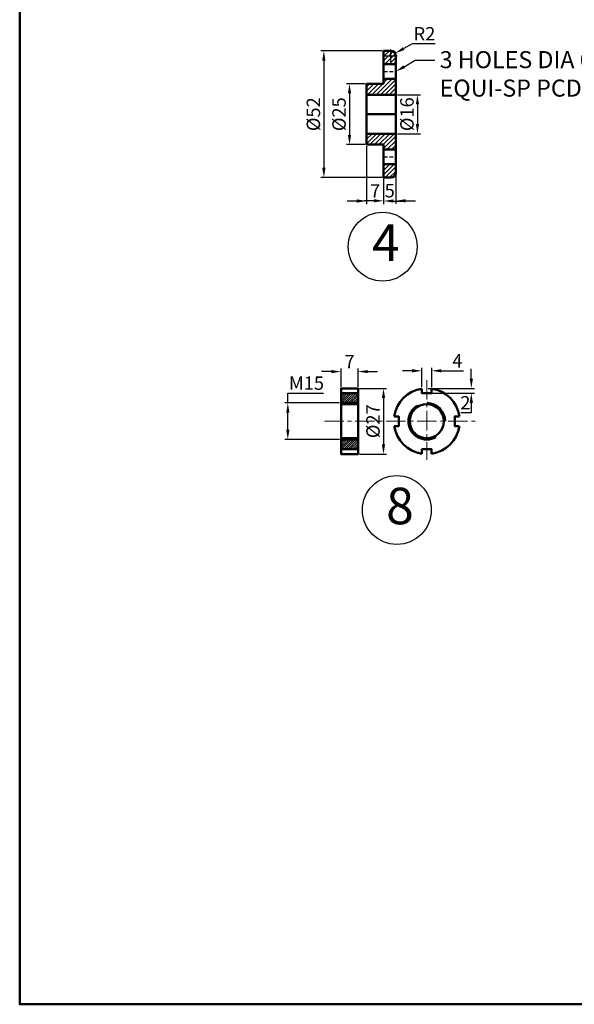
# Model space of a CAD drawing. Units: millimetres. Extents: x -3 to 930, y -425 to 322.
# Tile 1 of 5: x -3 to 225, y -425 to -21. Entities that reach past the tile are written whole.
import ezdxf
from ezdxf import colors
from ezdxf.entities.mleader import LeaderData, LeaderLine
from ezdxf.math import Vec2, Vec3

# ---------------------------------------------------------------- set-up
doc = ezdxf.new("R2010")
doc.units = ezdxf.units.MM
doc.header["$LTSCALE"] = 0.5
doc.linetypes.add('CENTER', pattern=[50.8, 31.75, -6.35, 6.35, -6.35])
doc.linetypes.add('HIDDEN', pattern=[9.525, 6.35, -3.175])
for name, color, linetype, lineweight in [('M-ANNO-SYMB', 3, 'Continuous', 25), ('M-CNTR', 1, 'CENTER', 18), ('M-DIMS', 2, 'Continuous', 25), ('M-HATC', 8, 'Continuous', 18), ('M-HIDN', 4, 'HIDDEN', 25), ('M-OUTL', 7, 'Continuous', 50), ('M-TEXT', 3, 'Continuous', 25)]:
    doc.layers.add(name, color=color, linetype=linetype, lineweight=lineweight)
doc.styles.get("Standard").update_dxf_attribs({"font": 'arial.ttf'})
doc.dimstyles.new('ISO-25', dxfattribs={"dimtxt": 5.5, "dimasz": 4, "dimexe": 1.25, "dimexo": 0.625, "dimtad": 1, "dimtoh": 1, "dimdec": 0, "dimtxsty": 'Standard', "dimcen": 2.5, "dimadec": 0, "dimazin": 0, "dimtfac": 1, "dimtdec": 0, "dimtofl": 0, "dimtmove": 0, "dimatfit": 3, "dimfxl": 1, "dimarcsym": 0})
pattern_1 = [(45, (-143.9728, 27.2126), (-0.8980256, 0.8980256), [])]

# ---------------------------------------------------------------- blocks, each defined once
blk = doc.blocks.new('*D43')
at = {"layer": 'Defpoints', "color": 0, "ltscale": 0.5, "transparency": 16777216}
for p in [(146.67, -33.61), (122.15, -85.61), (146.67, -85.61)]:
    blk.add_point(p, dxfattribs=at)
at = {"layer": 'M-DIMS', "color": 0, "lineweight": -2, "ltscale": 0.5, "transparency": 16777216}
for p, q in [((146.04, -33.61), (120.9, -33.61)), ((122.15, -37.61), (122.15, -81.61)), ((146.04, -85.61), (120.9, -85.61))]:
    blk.add_line(p, q, dxfattribs=at)
at = {"layer": 'M-DIMS', "color": 0, "ltscale": 0.5, "transparency": 16777216}
for points in [[(121.48, -37.61), (122.82, -37.61), (122.15, -33.61)], [(121.48, -81.61), (122.82, -81.61), (122.15, -85.61)]]:
    blk.add_solid(points, dxfattribs=at)
at = {"layer": 'M-DIMS', "color": 0, "ltscale": 0.5, "transparency": 16777216, "insert": (118.56, -59.61), "char_height": 5.5, "attachment_point": 5, "rotation": 90}
blk.add_mtext('%%C52', dxfattribs=at)
blk = doc.blocks.new('*D44')
at = {"layer": 'Defpoints', "color": 0, "ltscale": 0.5, "transparency": 16777216}
for p in [(139.67, -47.11), (132.67, -72.11), (139.67, -72.11)]:
    blk.add_point(p, dxfattribs=at)
at = {"layer": 'M-DIMS', "color": 0, "lineweight": -2, "ltscale": 0.5, "transparency": 16777216}
for p, q in [((139.04, -47.11), (131.42, -47.11)), ((132.67, -51.11), (132.67, -68.11)), ((139.04, -72.11), (131.42, -72.11))]:
    blk.add_line(p, q, dxfattribs=at)
at = {"layer": 'M-DIMS', "color": 0, "ltscale": 0.5, "transparency": 16777216}
for points in [[(132, -51.11), (133.34, -51.11), (132.67, -47.11)], [(132, -68.11), (133.34, -68.11), (132.67, -72.11)]]:
    blk.add_solid(points, dxfattribs=at)
at = {"layer": 'M-DIMS', "color": 0, "ltscale": 0.5, "transparency": 16777216, "insert": (129.08, -59.61), "char_height": 5.5, "attachment_point": 5, "rotation": 90}
blk.add_mtext('%%C25', dxfattribs=at)
blk = doc.blocks.new('*D45')
at = {"layer": 'Defpoints', "color": 0, "ltscale": 0.5, "transparency": 16777216}
for p in [(151.67, -51.61), (151.67, -67.61), (160.53, -67.61)]:
    blk.add_point(p, dxfattribs=at)
at = {"layer": 'M-DIMS', "color": 0, "lineweight": -2, "ltscale": 0.5, "transparency": 16777216}
for p, q in [((152.29, -51.61), (161.78, -51.61)), ((160.53, -55.61), (160.53, -63.61)), ((152.29, -67.61), (161.78, -67.61))]:
    blk.add_line(p, q, dxfattribs=at)
at = {"layer": 'M-DIMS', "color": 0, "ltscale": 0.5, "transparency": 16777216}
for points in [[(159.87, -55.61), (161.2, -55.61), (160.53, -51.61)], [(159.87, -63.61), (161.2, -63.61), (160.53, -67.61)]]:
    blk.add_solid(points, dxfattribs=at)
at = {"layer": 'M-DIMS', "color": 0, "ltscale": 0.5, "transparency": 16777216, "insert": (156.95, -59.61), "char_height": 5.5, "attachment_point": 5, "rotation": 90}
blk.add_mtext('%%C16', dxfattribs=at)
blk = doc.blocks.new('*D46')
at = {"layer": 'Defpoints', "color": 0, "ltscale": 0.5, "transparency": 16777216}
for p in [(139.67, -72.11), (146.67, -72.11), (146.67, -95.23)]:
    blk.add_point(p, dxfattribs=at)
at = {"layer": 'M-DIMS', "color": 0, "lineweight": -2, "ltscale": 0.5, "transparency": 16777216}
for p, q in [((139.67, -72.73), (139.67, -96.48)), ((146.67, -72.73), (146.67, -96.48)), ((135.67, -95.23), (131.67, -95.23)), ((150.67, -95.23), (154.67, -95.23))]:
    blk.add_line(p, q, dxfattribs=at)
at = {"layer": 'M-DIMS', "color": 0, "ltscale": 0.5, "transparency": 16777216}
for points in [[(135.67, -94.56), (135.67, -95.9), (139.67, -95.23)], [(150.67, -94.56), (150.67, -95.9), (146.67, -95.23)]]:
    blk.add_solid(points, dxfattribs=at)
at = {"layer": 'M-DIMS', "color": 0, "ltscale": 0.5, "transparency": 16777216, "insert": (143.17, -91.86), "char_height": 5.5, "attachment_point": 5}
blk.add_mtext('7', dxfattribs=at)
blk = doc.blocks.new('*D47')
at = {"layer": 'Defpoints', "color": 0, "ltscale": 0.5, "transparency": 16777216}
for p in [(146.67, -74.11), (151.67, -74.11), (151.67, -95.15)]:
    blk.add_point(p, dxfattribs=at)
at = {"layer": 'M-DIMS', "color": 0, "lineweight": -2, "ltscale": 0.5, "transparency": 16777216}
for p, q in [((146.67, -74.73), (146.67, -96.4)), ((151.67, -74.73), (151.67, -96.4)), ((142.67, -95.15), (138.67, -95.15)), ((155.67, -95.15), (159.67, -95.15))]:
    blk.add_line(p, q, dxfattribs=at)
at = {"layer": 'M-DIMS', "color": 0, "ltscale": 0.5, "transparency": 16777216}
for points in [[(142.67, -94.48), (142.67, -95.81), (146.67, -95.15)], [(155.67, -94.48), (155.67, -95.81), (151.67, -95.15)]]:
    blk.add_solid(points, dxfattribs=at)
at = {"layer": 'M-DIMS', "color": 0, "ltscale": 0.5, "transparency": 16777216, "insert": (149.17, -91.72), "char_height": 5.5, "attachment_point": 5}
blk.add_mtext('5', dxfattribs=at)
blk = doc.blocks.new('*D48')
at = {"layer": 'Defpoints', "color": 0, "ltscale": 0.5, "transparency": 16777216}
for p in [(149.67, -35.61), (151.41, -34.62)]:
    blk.add_point(p, dxfattribs=at)
at = {"layer": 'M-DIMS', "color": 0, "lineweight": -2, "ltscale": 0.5, "transparency": 16777216}
for p, q in [((158.38, -30.7), (154.89, -32.66)), ((167.82, -30.7), (158.38, -30.7)), ((147.17, -35.61), (152.17, -35.61)), ((149.67, -38.11), (149.67, -33.11))]:
    blk.add_line(p, q, dxfattribs=at)
at = {"layer": 'M-DIMS', "color": 0, "ltscale": 0.5, "transparency": 16777216}
blk.add_solid([(154.57, -32.08), (155.22, -33.24), (151.41, -34.62)], dxfattribs=at)
at = {"layer": 'M-DIMS', "color": 0, "ltscale": 0.5, "transparency": 16777216, "insert": (163.41, -27.31), "char_height": 5.5, "attachment_point": 5}
blk.add_mtext('R2', dxfattribs=at)
blk = doc.blocks.new('*D61')
at = {"layer": 'Defpoints', "color": 0, "ltscale": 0.5, "transparency": 16777216}
for p in [(107.36, -178.11), (129.18, -178.11), (129.18, -193.11)]:
    blk.add_point(p, dxfattribs=at)
at = {"layer": 'M-DIMS', "color": 0, "lineweight": -2, "ltscale": 0.5, "transparency": 16777216}
for p, q in [((107.36, -178.11), (107.36, -174.11)), ((107.36, -174.11), (122.06, -174.11)), ((128.56, -178.11), (106.11, -178.11)), ((107.36, -189.11), (107.36, -182.11)), ((128.56, -193.11), (106.11, -193.11))]:
    blk.add_line(p, q, dxfattribs=at)
at = {"layer": 'M-DIMS', "color": 0, "ltscale": 0.5, "transparency": 16777216}
for points in [[(106.7, -182.11), (108.03, -182.11), (107.36, -178.11)], [(106.7, -189.11), (108.03, -189.11), (107.36, -193.11)]]:
    blk.add_solid(points, dxfattribs=at)
at = {"layer": 'M-DIMS', "color": 0, "ltscale": 0.5, "transparency": 16777216, "insert": (115.02, -170.68), "char_height": 5.5, "attachment_point": 5}
blk.add_mtext('M15', dxfattribs=at)
blk = doc.blocks.new('*D62')
at = {"layer": 'Defpoints', "color": 0, "ltscale": 0.5, "transparency": 16777216}
for p in [(136.18, -165.24), (129.18, -172.11), (136.18, -172.11)]:
    blk.add_point(p, dxfattribs=at)
at = {"layer": 'M-DIMS', "color": 0, "lineweight": -2, "ltscale": 0.5, "transparency": 16777216}
for p, q in [((125.18, -165.24), (121.18, -165.24)), ((129.18, -171.49), (129.18, -163.99)), ((136.18, -171.49), (136.18, -163.99)), ((140.18, -165.24), (144.18, -165.24))]:
    blk.add_line(p, q, dxfattribs=at)
at = {"layer": 'M-DIMS', "color": 0, "ltscale": 0.5, "transparency": 16777216}
for points in [[(125.18, -164.57), (125.18, -165.9), (129.18, -165.24)], [(140.18, -164.57), (140.18, -165.9), (136.18, -165.24)]]:
    blk.add_solid(points, dxfattribs=at)
at = {"layer": 'M-DIMS', "color": 0, "ltscale": 0.5, "transparency": 16777216, "insert": (132.68, -161.86), "char_height": 5.5, "attachment_point": 5}
blk.add_mtext('7', dxfattribs=at)
blk = doc.blocks.new('*D63')
at = {"layer": 'Defpoints', "color": 0, "ltscale": 0.5, "transparency": 16777216}
for p in [(136.18, -172.11), (136.18, -199.11), (146.6, -199.11)]:
    blk.add_point(p, dxfattribs=at)
at = {"layer": 'M-DIMS', "color": 0, "lineweight": -2, "ltscale": 0.5, "transparency": 16777216}
for p, q in [((136.81, -172.11), (147.85, -172.11)), ((146.6, -176.11), (146.6, -195.11)), ((136.81, -199.11), (147.85, -199.11))]:
    blk.add_line(p, q, dxfattribs=at)
at = {"layer": 'M-DIMS', "color": 0, "ltscale": 0.5, "transparency": 16777216}
for points in [[(145.94, -176.11), (147.27, -176.11), (146.6, -172.11)], [(145.94, -195.11), (147.27, -195.11), (146.6, -199.11)]]:
    blk.add_solid(points, dxfattribs=at)
at = {"layer": 'M-DIMS', "color": 0, "ltscale": 0.5, "transparency": 16777216, "insert": (143.02, -185.61), "char_height": 5.5, "attachment_point": 5, "rotation": 90}
blk.add_mtext('%%C27', dxfattribs=at)
blk = doc.blocks.new('*D64')
at = {"layer": 'Defpoints', "color": 0, "ltscale": 0.5, "transparency": 16777216}
for p in [(166.37, -164.91), (162.37, -172.26), (166.37, -172.26)]:
    blk.add_point(p, dxfattribs=at)
at = {"layer": 'M-DIMS', "color": 0, "lineweight": -2, "ltscale": 0.5, "transparency": 16777216}
for p, q in [((158.37, -164.91), (154.37, -164.91)), ((162.37, -171.64), (162.37, -163.66)), ((166.37, -171.64), (166.37, -163.66)), ((170.37, -164.91), (179.42, -164.91))]:
    blk.add_line(p, q, dxfattribs=at)
at = {"layer": 'M-DIMS', "color": 0, "ltscale": 0.5, "transparency": 16777216}
for points in [[(158.37, -164.24), (158.37, -165.57), (162.37, -164.91)], [(170.37, -164.24), (170.37, -165.57), (166.37, -164.91)]]:
    blk.add_solid(points, dxfattribs=at)
at = {"layer": 'M-DIMS', "color": 0, "ltscale": 0.5, "transparency": 16777216, "insert": (176.9, -161.53), "char_height": 5.5, "attachment_point": 5}
blk.add_mtext('4', dxfattribs=at)
blk = doc.blocks.new('*D65')
at = {"layer": 'Defpoints', "color": 0, "ltscale": 0.5, "transparency": 16777216}
for p in [(164.37, -172.11), (164.37, -174.11), (182.63, -174.11)]:
    blk.add_point(p, dxfattribs=at)
at = {"layer": 'M-DIMS', "color": 0, "lineweight": -2, "ltscale": 0.5, "transparency": 16777216}
for p, q in [((182.63, -168.11), (182.63, -164.11)), ((164.99, -172.11), (183.88, -172.11)), ((164.99, -174.11), (183.88, -174.11)), ((182.63, -178.11), (182.63, -182.11)), ((182.63, -182.11), (178.36, -182.11))]:
    blk.add_line(p, q, dxfattribs=at)
at = {"layer": 'M-DIMS', "color": 0, "ltscale": 0.5, "transparency": 16777216}
for points in [[(181.97, -168.11), (183.3, -168.11), (182.63, -172.11)], [(181.97, -178.11), (183.3, -178.11), (182.63, -174.11)]]:
    blk.add_solid(points, dxfattribs=at)
at = {"layer": 'M-DIMS', "color": 0, "ltscale": 0.5, "transparency": 16777216, "insert": (180.19, -178.73), "char_height": 5.5, "attachment_point": 5}
blk.add_mtext('2', dxfattribs=at)
blk = doc.blocks.new('BALLOON')
at = {"ltscale": 0.5}
blk.add_circle((198.15, 8.03), 14.13, dxfattribs=at)
blk = doc.blocks.new('NUT-END-VIEW')
at = {"ltscale": 0.5}
for points in [[(15.35, 26.7), (15.35, 24.85), (11.35, 24.85), (11.35, 26.7)], [(0, 15.35), (1.85, 15.35), (1.85, 11.35), (0, 11.35)], [(26.7, 11.35), (24.85, 11.35), (24.85, 15.35), (26.7, 15.35)], [(11.35, 0), (11.35, 1.85), (15.35, 1.85), (15.35, 0)]]:
    blk.add_lwpolyline(points, dxfattribs=at)
for start, end in [(98.5196, 171.4804), (8.5196, 81.4804), (188.5196, 261.4804), (278.5196, 351.4804)]:
    blk.add_arc((13.35, 13.35), 13.5, start, end, dxfattribs=at)

msp = doc.modelspace()

# ---------------------------------------------------------------- hatches: boundary and pattern name
at = {"layer": 'M-HATC', "ltscale": 0.5}
h = msp.add_hatch(dxfattribs=at)
h.set_pattern_fill('ANSI31', color=256, scale=0.4)
h.set_pattern_definition(pattern_1)
h.paths.add_polyline_path([(146.6663, -39.1062), (151.6663, -39.1062), (151.6663, -35.6062, 0.41421356), (149.6663, -33.6062), (146.6663, -33.6062)])
h.paths.add_polyline_path([(146.6663, -80.1062), (146.6663, -85.6062), (149.6663, -85.6062, 0.41421356), (151.6663, -83.6062), (151.6663, -80.1062)])
h = msp.add_hatch(dxfattribs=at)
h.set_pattern_fill('ANSI31', color=256, scale=0.4)
h.set_pattern_definition(pattern_1)
h.paths.add_polyline_path([(151.6663, -45.1062), (146.6663, -45.1062), (146.6663, -47.1062), (139.6663, -47.1062), (139.6663, -51.6062), (151.6663, -51.6062)])
h.paths.add_polyline_path([(151.6663, -67.6062), (139.6663, -67.6062), (139.6663, -72.1062), (146.6663, -72.1062), (146.6663, -74.1062), (151.6663, -74.1062)])
h = msp.add_hatch(dxfattribs=at)
h.set_pattern_fill('ANSI31', color=256, scale=0.2)
h.set_pattern_definition([(45, (-261.27354, -62.43613), (-0.4490128, 0.4490128), [])])
h.paths.add_polyline_path([(136.1835, -174.1121), (129.1835, -174.1121), (129.1835, -178.1121), (136.1835, -178.1121)])
h.paths.add_polyline_path([(136.1835, -193.1121), (129.1835, -193.1121), (129.1835, -197.1121), (136.1835, -197.1121)])

# ---------------------------------------------------------------- linework, layer by layer
at = {"layer": 'M-CNTR', "ltscale": 0.5}
for p, q in [((164.3687, -168.7049), (164.3687, -201.5017)), ((122.3431, -185.6121), (184.8222, -185.6121))]:
    msp.add_line(p, q, dxfattribs=at)
at = {"layer": 'M-HIDN', "ltscale": 0.5}
for p, q in [((146.6663, -42.1062), (151.6663, -42.1062)), ((146.6663, -77.1062), (151.6663, -77.1062))]:
    msp.add_line(p, q, dxfattribs=at)
at = {"layer": 'M-OUTL', "ltscale": 0.5}
for p, q in [((146.6663, -33.6062), (149.6663, -33.6062)), ((146.6663, -33.6062), (146.6663, -47.1062)), ((151.6663, -35.6062), (151.6663, -83.6062)), ((146.6663, -39.1062), (151.6663, -39.1062)), ((139.6663, -72.1062), (139.6663, -47.1062)), ((139.6663, -47.1062), (146.6663, -47.1062)), ((146.6663, -45.1062), (151.6663, -45.1062)), ((139.6663, -51.6062), (151.6663, -51.6062)), ((139.6663, -59.6062), (151.6663, -59.6062)), ((139.6663, -67.6062), (151.6663, -67.6062)), ((139.6663, -72.1062), (146.6663, -72.1062)), ((146.6663, -72.1062), (146.6663, -85.6062)), ((146.6663, -74.1062), (151.6663, -74.1062)), ((146.6663, -80.1062), (151.6663, -80.1062)), ((149.6663, -85.6062), (146.6663, -85.6062)), ((136.1835, -174.1121), (129.1835, -174.1121)), ((136.1835, -178.1121), (129.1835, -178.1121)), ((136.1835, -178.6121), (129.1835, -178.6121)), ((160.8687, -179.5499), (160.6187, -179.1169)), ((136.1835, -192.6121), (129.1835, -192.6121)), ((136.1835, -193.1121), (129.1835, -193.1121)), ((168.1187, -192.1073), (167.8687, -191.6743)), ((136.1835, -197.1121), (129.1835, -197.1121))]:
    msp.add_line(p, q, dxfattribs=at)
for points in [[(-2.6134, 321.6785), (929.6113, 321.6785), (929.6113, -424.8872), (-2.6134, -424.8872)], [(136.1835, -199.1121), (136.1835, -185.6121), (136.1835, -172.1121), (129.1835, -172.1121), (129.1835, -199.1121)]]:
    msp.add_lwpolyline(points, close=True, dxfattribs=at)
msp.add_circle((164.3687, -185.6121), 7, dxfattribs=at)
for centre, radius, start, end in [((149.6663, -35.6062), 2, 0, 90), ((149.6663, -83.6062), 2, 270, 0), ((164.3687, -185.6121), 7.5, 120, 300), ((164.3687, -185.6121), 7.5, 0, 90)]:
    msp.add_arc(centre, radius, start, end, dxfattribs=at)

# ---------------------------------------------------------------- block references
at = {"layer": 'M-ANNO-SYMB'}
for p in [(-51.8624, -121.9964), (-46.0696, -230.0888)]:
    msp.add_blockref('BALLOON', p, dxfattribs=at)
at = {"layer": 'M-OUTL'}
msp.add_blockref('NUT-END-VIEW', (151.018, -198.963), dxfattribs=at)

# ---------------------------------------------------------------- texts
at = {"layer": 'M-TEXT', "ltscale": 0.5, "char_height": 15, "attachment_point": 1}
for s, insert in [('4', (141.8894, -104.788)), ('8', (147.6822, -212.8804))]:
    msp.add_mtext_dynamic_manual_height_columns(s, width=15, gutter_width=12.5, heights=[0], dxfattribs=dict(at, insert=insert))

# ---------------------------------------------------------------- dimensions: what is measured, and where the dimension line sits
at = {"layer": 'M-DIMS', "ltscale": 0.5}
dim = msp.add_radius_dim(center=(149.6663, -35.6062), mpoint=(151.4087, -34.6243), dimstyle='ISO-25', override={"dimclrd": 0, "dimclre": 0, "dimclrt": 0}, dxfattribs=at)
dim.commit()
dim.dimension.update_dxf_attribs({"geometry": '*D48', "text_midpoint": (163.4097, -27.3106)})
for base, p1, p2, picture, middle in [((122.1512, -85.6062), (146.6663, -33.6062), (146.6663, -85.6062), '*D43', (118.5642, -59.6062)), ((132.6713, -72.1062), (139.6663, -47.1062), (139.6663, -72.1062), '*D44', (129.0843, -59.6062)), ((160.5344, -67.6062), (151.6663, -51.6062), (151.6663, -67.6062), '*D45', (156.9474, -59.6062)), ((146.6037, -199.1121), (136.1835, -172.1121), (136.1835, -199.1121), '*D63', (143.0167, -185.6121))]:
    dim = msp.add_linear_dim(base=base, p1=p1, p2=p2, angle=90, text='%%C<>', dimstyle='ISO-25', override={"dimclrd": 0, "dimclre": 0, "dimclrt": 0}, dxfattribs=at)
    dim.commit()
    dim.dimension.update_dxf_attribs({"geometry": picture, "text_midpoint": middle})
for base, p1, p2, picture, middle in [((146.6663, -95.2301), (139.6663, -72.1062), (146.6663, -72.1062), '*D46', (143.1663, -91.8551)), ((151.6663, -95.1453), (146.6663, -74.1062), (151.6663, -74.1062), '*D47', (149.1663, -91.7234)), ((136.1835, -165.2359), (129.1835, -172.1121), (136.1835, -172.1121), '*D62', (132.6835, -161.8609)), ((166.3687, -164.9064), (162.3687, -172.2611), (166.3687, -172.2611), '*D64', (176.8958, -161.5314))]:
    dim = msp.add_linear_dim(base=base, p1=p1, p2=p2, dimstyle='ISO-25', override={"dimclrd": 0, "dimclre": 0, "dimclrt": 0}, dxfattribs=at)
    dim.commit()
    dim.dimension.update_dxf_attribs({"geometry": picture, "text_midpoint": middle})
dim = msp.add_linear_dim(base=(182.6322, -174.1121), p1=(164.3687, -172.1121), p2=(164.3687, -174.1121), angle=90, dimstyle='ISO-25', override={"dimclrd": 0, "dimclre": 0, "dimclrt": 0}, dxfattribs=at)
dim.commit()
dim.dimension.update_dxf_attribs({"geometry": '*D65', "text_midpoint": (180.1857, -178.7258)})
dim = msp.add_linear_dim(base=(107.3636, -178.1121), p1=(129.1835, -193.1121), p2=(129.1835, -178.1121), angle=90, text='M<>', dimstyle='ISO-25', override={"dimclrd": 0, "dimclre": 0, "dimclrt": 0}, dxfattribs=at)
dim.commit()
dim.dimension.update_dxf_attribs({"geometry": '*D61', "text_midpoint": (115.023, -174.1121), "dimtype": 160})

# ---------------------------------------------------------------- leaders
ml = msp.add_multileader_mtext('Standard', dxfattribs=at)
ml.set_content('3 HOLES DIA 6\\PEQUI-SP PCD 35', color=256)
ml.set_leader_properties()
ml.build(insert=Vec2(0, 0))
ctx = ml.context
ctx.base_point, ctx.char_height, ctx.plane_origin = Vec3(167.6494, -37.4972), 7, Vec3(151.6663, -42.1062)
notes = []
notes.append((ctx, [(1, (1, 1, 0), (159.6494, -37.4972), (1, 0), 8, [(0, [(151.6663, -42.1062)], 0, [])])]))
ctx.mtext.insert, ctx.mtext.flow_direction = Vec3(169.6494, -33.7251), 5
for ctx, leaders in notes:
    for number, flags, end, landing, length, lines in leaders:
        leader = LeaderData()
        leader.index, (leader.has_last_leader_line, leader.has_dogleg_vector, leader.attachment_direction) = number, flags
        leader.last_leader_point, leader.dogleg_vector, leader.dogleg_length = Vec3(end), Vec3(landing), length
        for number, points, colour, breaks in lines:
            line = LeaderLine()
            line.index, line.vertices, line.color, line.breaks = number, Vec3.list(points), colors.encode_raw_color(colour), breaks
            leader.lines.append(line)
        ctx.leaders.append(leader)

doc.saveas('drawing.dxf')
